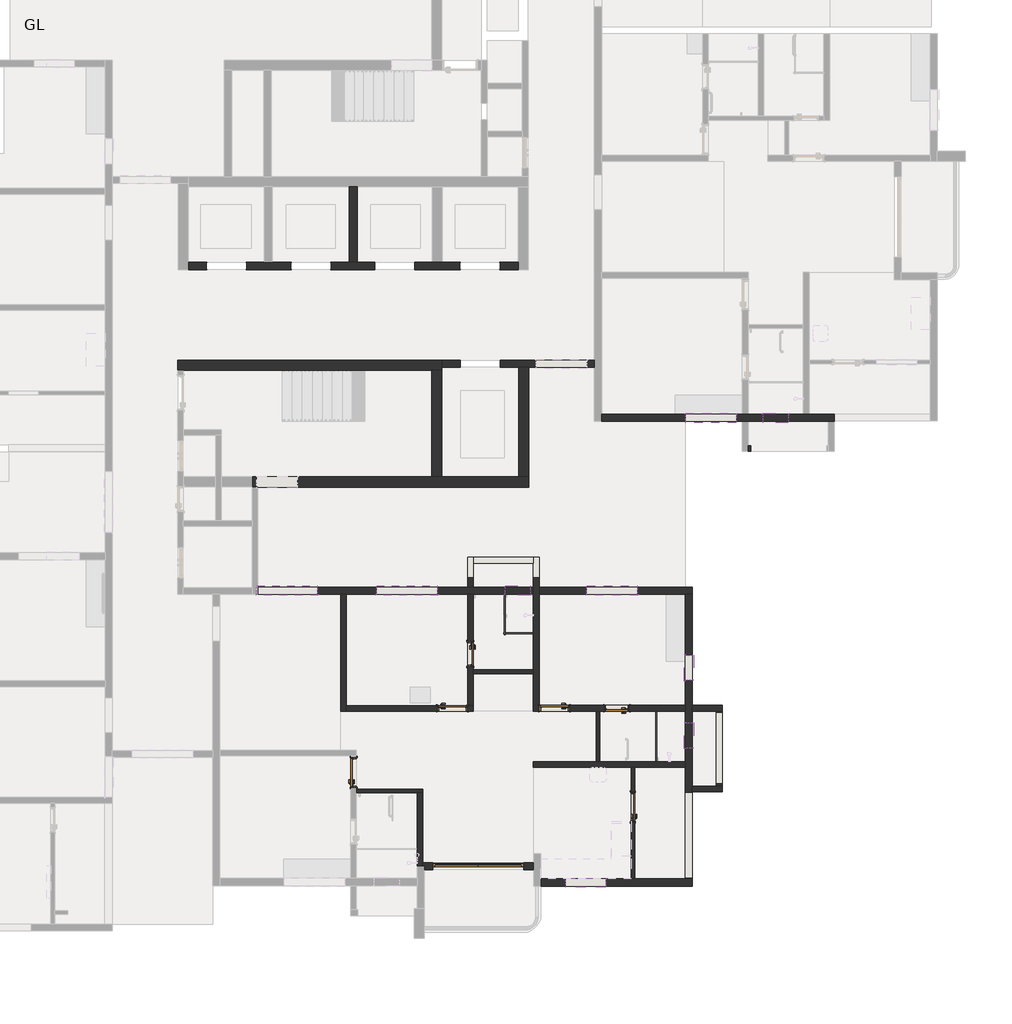
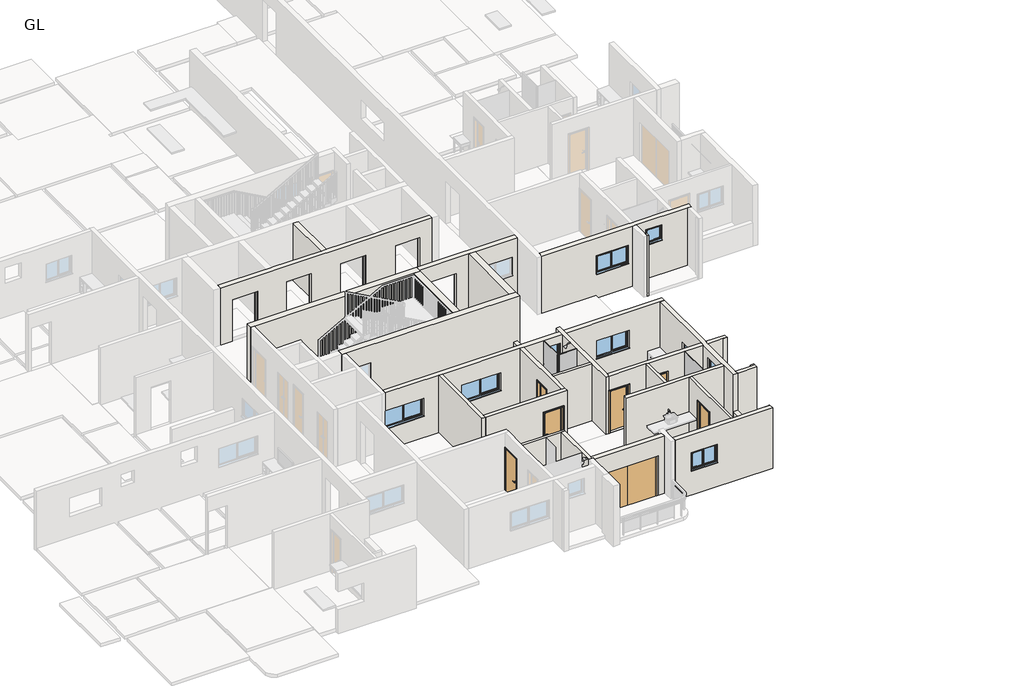
# One storey, part 4 of 14: 35 walls, 9 windows, 7 doors, 3 plates.
"""IFC4 building model written with IfcOpenShell, lengths in millimetres."""

from ifc_helpers import new_model, si_unit, frame, origin, origin_with_axes, place, context, project, spatial, polyline, outline, extrude, faceted_brep, transform, mapped, element, save
from components import doors_concept_extdbl_9_dbcc4ac8, doors_intsgl_2_5_door_ce04bd24, doors_intsgl_3_door_8261d8fb, doors_intsgl_3_door_f61d7fb9, doors_intsgl_3_door_feb48a3d, doors_intsgl_3_door_d2de26da, system_panel_glazed_00f127ae, system_panel_glazed_ff4fe8f0, system_panel_glazed_94d7f8cb, windows_dbl_plain_2_5_f94f9a84, windows_dbl_plain_4_905afcad, windows_dbl_plain_5_907a13a5, windows_dbl_plain_6_3da2432f, windows_sgl_plain_2_5_21186da1

model = new_model("IFC4")

# Units and contexts
model_context = context("Model", 3, world=origin())
ifc_project = project(units=[si_unit("LENGTHUNIT", "METRE", prefix="MILLI")], contexts=[model_context])

# Site, building, storey
site = spatial("IfcSite", under=ifc_project)
building = spatial("IfcBuilding", under=site)
storey = spatial("IfcBuildingStorey", under=building, Name="GL", Elevation=0.0)

# Doors
placement = place(None, origin())
doors_concept_extdbl_9_shape = doors_concept_extdbl_9_dbcc4ac8(model_context)
element("IfcDoor", 1, ObjectType="Doors_Concept_ExtDbl : 9'", at=placement, inside=storey, context=model_context, shape_type="MappedRepresentation", body=[
    mapped(doors_concept_extdbl_9_shape, transform((5777.5463567, 58086.1033045, 0.0), x_axis=(1.0, 0.0, 0.0), y_axis=(0.0, 1.0, 0.0), z_axis=(0.0, 0.0, 1.0))),
])
doors_intsgl_2_5_door_shape = doors_intsgl_2_5_door_ce04bd24(model_context)
element("IfcDoor", 2, ObjectType="Doors_IntSgl : 2.5' DOOR", at=placement, inside=storey, context=model_context, shape_type="MappedRepresentation", body=[
    mapped(doors_intsgl_2_5_door_shape, transform((5542.845694, 64510.7496197, 149.9616), x_axis=(0.0, -1.0, 0.0), y_axis=(1.0, 0.0, 0.0), z_axis=(0.0, 0.0, 1.0))),
])
element("IfcDoor", 3, ObjectType="Doors_IntSgl : 2.5' DOOR", at=placement, inside=storey, context=model_context, shape_type="MappedRepresentation", body=[
    mapped(doors_intsgl_2_5_door_shape, transform((9968.9401818, 62868.569994, 149.9616), x_axis=(-1.0, 0.0, 0.0), y_axis=(0.0, -1.0, 0.0), z_axis=(0.0, 0.0, 1.0))),
])
doors_intsgl_3_door_shape = doors_intsgl_3_door_8261d8fb(model_context)
element("IfcDoor", 4, ObjectType="Doors_IntSgl : 3' DOOR", at=placement, inside=storey, context=model_context, shape_type="MappedRepresentation", body=[
    mapped(doors_intsgl_3_door_shape, transform((8080.813694, 62868.569994, 149.9616), x_axis=(-1.0, 0.0, 0.0), y_axis=(0.0, -1.0, 0.0), z_axis=(0.0, 0.0, 1.0))),
])
doors_intsgl_3_door_2_shape = doors_intsgl_3_door_f61d7fb9(model_context)
element("IfcDoor", 5, ObjectType="Doors_IntSgl : 3' DOOR", at=placement, inside=storey, context=model_context, shape_type="MappedRepresentation", body=[
    mapped(doors_intsgl_3_door_2_shape, transform((4998.777694, 62865.3348421, 149.9616), x_axis=(1.0, 0.0, 0.0), y_axis=(0.0, 1.0, 0.0), z_axis=(0.0, 0.0, 1.0))),
])
doors_intsgl_3_door_3_shape = doors_intsgl_3_door_feb48a3d(model_context)
element("IfcDoor", 6, ObjectType="Doors_IntSgl : 3' DOOR", at=placement, inside=storey, context=model_context, shape_type="MappedRepresentation", body=[
    mapped(doors_intsgl_3_door_3_shape, transform((2014.4093567, 60927.6425384, 149.9616), x_axis=(0.0, 1.0, 0.0), y_axis=(-1.0, 0.0, 0.0), z_axis=(0.0, 0.0, 1.0))),
])
doors_intsgl_3_door_4_shape = doors_intsgl_3_door_d2de26da(model_context)
element("IfcDoor", 7, ObjectType="Doors_IntSgl : 3' DOOR", at=placement, inside=storey, context=model_context, shape_type="MappedRepresentation", body=[
    mapped(doors_intsgl_3_door_4_shape, transform((10458.253694, 59886.101994, 149.9616), x_axis=(0.0, 1.0, 0.0), y_axis=(-1.0, 0.0, 0.0), z_axis=(0.0, 0.0, 1.0))),
])

# Plates
system_panel_glazed_shape = system_panel_glazed_00f127ae(model_context)
element("IfcPlate", 8, ObjectType="System Panel : Glazed", at=placement, inside=storey, context=model_context, shape_type="MappedRepresentation", body=[
    mapped(system_panel_glazed_shape, transform((6544.913694, 65695.8028421, 0.0), x_axis=(0.0, -1.0, 0.0), y_axis=(1.0, 0.0, 0.0), z_axis=(0.0, 0.0, 1.0))),
])
system_panel_glazed_2_shape = system_panel_glazed_ff4fe8f0(model_context)
element("IfcPlate", 9, ObjectType="System Panel : Glazed", at=placement, inside=storey, context=model_context, shape_type="MappedRepresentation", body=[
    mapped(system_panel_glazed_2_shape, transform((6997.395694, 65098.9028421, 0.0), x_axis=(1.0, 0.0, 0.0), y_axis=(0.0, 1.0, 0.0), z_axis=(0.0, 0.0, 1.0))),
])
system_panel_glazed_3_shape = system_panel_glazed_94d7f8cb(model_context)
element("IfcPlate", 10, ObjectType="System Panel : Glazed", at=placement, inside=storey, context=model_context, shape_type="MappedRepresentation", body=[
    mapped(system_panel_glazed_3_shape, transform((11125.003694, 62017.669994, 0.0), x_axis=(0.0, -1.0, 0.0), y_axis=(1.0, 0.0, 0.0), z_axis=(0.0, 0.0, 1.0))),
])

# Walls
element("IfcWall", 11, ObjectType="W2", at=placement, inside=storey, context=model_context, shape_type="SweptSolid", body=[
    extrude(outline(polyline([(13943.8163556, 70812.6678957), (14020.0163556, 70812.6678957), (14020.0163556, 70638.9318957), (13943.8163556, 70638.9318957), (13943.8163556, 70812.6678957)])), origin_with_axes(), (0.0, 0.0, 1.0), 3000.0),
])
element("IfcWall", 12, ObjectType="W2", at=placement, inside=storey, context=model_context, shape_type="Brep", body=[
    faceted_brep([(3929.8233567, 60310.5083045, 0.0), (3929.8233567, 58086.1033045, 0.0), (3929.8233567, 58086.1033045, 3000.0), (3929.8233567, 60310.5083045, 3000.0), (4103.5593567, 60310.5083045, 0.0), (4103.5593567, 60310.5083045, 3000.0), (4103.5593567, 58192.7833045, 3000.0), (4103.5593567, 58086.1033045, 3000.0), (4103.5593567, 58086.1033045, 0.0), (4103.5593567, 58192.7833045, 0.0)], [[[0, 1, 2, 3]], [[4, 5, 6, 7, 8, 9]], [[1, 0, 4, 9, 8]], [[2, 1, 8, 7]], [[3, 2, 7, 6, 5]], [[0, 3, 5, 4]]]),
])
element("IfcWall", 13, ObjectType="W2", at=placement, inside=storey, context=model_context, shape_type="Brep", body=[
    faceted_brep([(1620.577694, 66317.7028421, 0.0), (1620.577694, 62778.4668421, 0.0), (1620.577694, 62778.4668421, 3000.0), (1620.577694, 66317.7028421, 3000.0), (1794.313694, 66317.7028421, 0.0), (1794.313694, 66317.7028421, 3000.0), (1794.313694, 62952.2028421, 3000.0), (1794.313694, 62778.4668421, 3000.0), (1794.313694, 62778.4668421, 0.0), (1794.313694, 62952.2028421, 0.0)], [[[0, 1, 2, 3]], [[4, 5, 6, 7, 8, 9]], [[1, 0, 4, 9, 8]], [[3, 2, 7, 6, 5]], [[0, 3, 5, 4]], [[2, 1, 8, 7]]]),
])
element("IfcWall", 14, ObjectType="W2", at=placement, inside=storey, context=model_context, shape_type="Brep", body=[
    faceted_brep([(1794.313694, 62778.4668421, 0.0), (5629.713694, 62778.4668421, 0.0), (5629.713694, 62778.4668421, 3000.0), (1794.313694, 62778.4668421, 3000.0), (5455.977694, 62778.4668421, 2259.9616), (5455.977694, 62778.4668421, 149.9616), (4541.577694, 62778.4668421, 149.9616), (4541.577694, 62778.4668421, 2259.9616), (5629.713694, 62952.2028421, 0.0), (5455.977694, 62952.2028421, 0.0), (1794.313694, 62952.2028421, 0.0), (1794.313694, 62952.2028421, 3000.0), (5455.977694, 62952.2028421, 3000.0), (5629.713694, 62952.2028421, 3000.0), (5455.977694, 62952.2028421, 149.9616), (5455.977694, 62952.2028421, 2259.9616), (4541.577694, 62952.2028421, 2259.9616), (4541.577694, 62952.2028421, 149.9616)], [[[0, 1, 2, 3], [4, 5, 6, 7]], [[8, 9, 10, 11, 12, 13], [14, 15, 16, 17]], [[1, 0, 10, 9, 8]], [[3, 2, 13, 12, 11]], [[0, 3, 11, 10]], [[2, 1, 8, 13]], [[14, 5, 4, 15]], [[15, 4, 7, 16]], [[16, 7, 6, 17]], [[5, 14, 17, 6]]]),
])
element("IfcWall", 15, ObjectType="W2", at=placement, inside=storey, context=model_context, shape_type="Brep", body=[
    faceted_brep([(5629.713694, 62952.2028421, 0.0), (5629.713694, 63913.8496197, 0.0), (5629.713694, 64028.1496197, 0.0), (5629.713694, 66317.7028421, 0.0), (5629.713694, 66317.7028421, 3000.0), (5629.713694, 64028.1496197, 3000.0), (5629.713694, 63913.8496197, 3000.0), (5629.713694, 62952.2028421, 3000.0), (5629.713694, 64129.7496197, 149.9616), (5629.713694, 64129.7496197, 2259.9616), (5629.713694, 64891.7496197, 2259.9616), (5629.713694, 64891.7496197, 149.9616), (5455.977694, 66317.7028421, 0.0), (5455.977694, 62952.2028421, 0.0), (5455.977694, 62952.2028421, 149.9616), (5455.977694, 62952.2028421, 2259.9616), (5455.977694, 62952.2028421, 3000.0), (5455.977694, 66317.7028421, 3000.0), (5455.977694, 64129.7496197, 2259.9616), (5455.977694, 64129.7496197, 149.9616), (5455.977694, 64891.7496197, 149.9616), (5455.977694, 64891.7496197, 2259.9616)], [[[0, 1, 2, 3, 4, 5, 6, 7], [8, 9, 10, 11]], [[12, 13, 14, 15, 16, 17], [18, 19, 20, 21]], [[3, 2, 1, 0, 13, 12]], [[7, 6, 5, 4, 17, 16]], [[0, 7, 16, 15, 14, 13]], [[4, 3, 12, 17]], [[8, 19, 18, 9]], [[9, 18, 21, 10]], [[10, 21, 20, 11]], [[19, 8, 11, 20]]]),
])
element("IfcWall", 16, ObjectType="W2", at=placement, inside=storey, context=model_context, shape_type="Brep", body=[
    faceted_brep([(5629.713694, 66531.0628421, 0.0), (5629.713694, 66823.1628421, 0.0), (5629.713694, 66823.1628421, 561.6), (5629.713694, 66823.1628421, 3000.0), (5629.713694, 66531.0628421, 3000.0), (5455.977694, 66531.0628421, 0.0), (5455.977694, 66531.0628421, 3000.0), (5455.977694, 66823.1628421, 3000.0), (5455.977694, 66823.1628421, 561.6), (5455.977694, 66823.1628421, 0.0)], [[[0, 1, 2, 3, 4]], [[5, 6, 7, 8, 9]], [[1, 0, 5, 9]], [[3, 2, 1, 9, 8, 7]], [[4, 3, 7, 6]], [[0, 4, 6, 5]]]),
])
element("IfcWall", 17, ObjectType="W2", at=placement, inside=storey, context=model_context, shape_type="Brep", body=[
    faceted_brep([(7623.613694, 62781.701994, 0.0), (7623.613694, 62955.437994, 0.0), (7623.613694, 66823.1628421, 0.0), (7623.613694, 66823.1628421, 561.6), (7623.613694, 66823.1628421, 3000.0), (7623.613694, 62955.437994, 3000.0), (7623.613694, 62781.701994, 3000.0), (7623.613694, 62781.701994, 2259.9616), (7623.613694, 62781.701994, 149.9616), (7449.877694, 62781.701994, 0.0), (7449.877694, 62781.701994, 3000.0), (7449.877694, 63913.8496197, 3000.0), (7449.877694, 64028.1496197, 3000.0), (7449.877694, 66823.1628421, 3000.0), (7449.877694, 66823.1628421, 561.6), (7449.877694, 66823.1628421, 0.0), (7449.877694, 64028.1496197, 0.0), (7449.877694, 63913.8496197, 0.0)], [[[0, 1, 2, 3, 4, 5, 6, 7, 8]], [[9, 10, 11, 12, 13, 14, 15, 16, 17]], [[2, 1, 0, 9, 17, 16, 15]], [[4, 3, 2, 15, 14, 13]], [[6, 5, 4, 13, 12, 11, 10]], [[0, 8, 7, 6, 10, 9]]]),
])
element("IfcWall", 18, ObjectType="W2", at=placement, inside=storey, context=model_context, shape_type="SweptSolid", body=[
    extrude(outline(polyline([(7449.877694, 67257.1218421), (5629.713694, 67257.1218421), (5629.713694, 67430.8578421), (7449.877694, 67430.8578421), (7449.877694, 67257.1218421)])), origin_with_axes(), (0.0, 0.0, 1.0), 561.6),
])
element("IfcWall", 19, ObjectType="W2", at=placement, inside=storey, context=model_context, shape_type="Brep", body=[
    faceted_brep([(5629.713694, 66823.1628421, 0.0), (5629.713694, 67257.1218421, 0.0), (5629.713694, 67430.8578421, 0.0), (5629.713694, 67430.8578421, 561.6), (5629.713694, 67257.1218421, 561.6), (5629.713694, 66823.1628421, 561.6), (5455.977694, 66823.1628421, 0.0), (5455.977694, 66823.1628421, 561.6), (5455.977694, 67430.8578421, 561.6), (5455.977694, 67430.8578421, 0.0)], [[[0, 1, 2, 3, 4, 5]], [[6, 7, 8, 9]], [[2, 1, 0, 6, 9]], [[5, 4, 3, 8, 7]], [[0, 5, 7, 6]], [[3, 2, 9, 8]]]),
])
element("IfcWall", 20, ObjectType="W2", at=placement, inside=storey, context=model_context, shape_type="Brep", body=[
    faceted_brep([(7623.613694, 66823.1628421, 0.0), (7623.613694, 67430.8578421, 0.0), (7623.613694, 67430.8578421, 561.6), (7623.613694, 66823.1628421, 561.6), (7449.877694, 66823.1628421, 0.0), (7449.877694, 66823.1628421, 561.6), (7449.877694, 67257.1218421, 561.6), (7449.877694, 67430.8578421, 561.6), (7449.877694, 67430.8578421, 0.0), (7449.877694, 67257.1218421, 0.0)], [[[0, 1, 2, 3]], [[4, 5, 6, 7, 8, 9]], [[1, 0, 4, 9, 8]], [[3, 2, 7, 6, 5]], [[0, 3, 5, 4]], [[2, 1, 8, 7]]]),
])
element("IfcWall", 21, ObjectType="W2", at=placement, inside=storey, context=model_context, shape_type="Brep", body=[
    faceted_brep([(12252.763694, 60342.3528421, 0.0), (13154.463694, 60342.3528421, 0.0), (13154.463694, 60342.3528421, 3000.0), (12252.763694, 60342.3528421, 3000.0), (12252.763694, 60516.0888421, 0.0), (12252.763694, 60516.0888421, 3000.0), (12980.727694, 60516.0888421, 3000.0), (13154.463694, 60516.0888421, 3000.0), (13154.463694, 60516.0888421, 0.0), (12980.727694, 60516.0888421, 0.0)], [[[0, 1, 2, 3]], [[4, 5, 6, 7, 8, 9]], [[1, 0, 4, 9, 8]], [[3, 2, 7, 6, 5]], [[2, 1, 8, 7]], [[0, 3, 5, 4]]]),
])
element("IfcWall", 22, ObjectType="W2", at=placement, inside=storey, context=model_context, shape_type="Brep", body=[
    faceted_brep([(12252.763694, 62781.701994, 0.0), (12980.727694, 62781.701994, 0.0), (13154.463694, 62781.701994, 0.0), (13154.463694, 62781.701994, 3000.0), (12980.727694, 62781.701994, 3000.0), (12252.763694, 62781.701994, 3000.0), (12252.763694, 62955.437994, 0.0), (12252.763694, 62955.437994, 3000.0), (13154.463694, 62955.437994, 3000.0), (13154.463694, 62955.437994, 0.0)], [[[0, 1, 2, 3, 4, 5]], [[6, 7, 8, 9]], [[2, 1, 0, 6, 9]], [[5, 4, 3, 8, 7]], [[0, 5, 7, 6]], [[3, 2, 9, 8]]]),
])
element("IfcWall", 23, ObjectType="W2", at=placement, inside=storey, context=model_context, shape_type="Brep", body=[
    faceted_brep([(13154.463694, 60516.0888421, 0.0), (13154.463694, 60592.2888421, 0.0), (13154.463694, 60592.2888421, 1171.2), (13154.463694, 60592.2888421, 3000.0), (13154.463694, 60516.0888421, 3000.0), (12980.727694, 60516.0888421, 0.0), (12980.727694, 60516.0888421, 3000.0), (12980.727694, 60592.2888421, 3000.0), (12980.727694, 60592.2888421, 1171.2), (12980.727694, 60592.2888421, 0.0)], [[[0, 1, 2, 3, 4]], [[5, 6, 7, 8, 9]], [[1, 0, 5, 9]], [[3, 2, 1, 9, 8, 7]], [[4, 3, 7, 6]], [[0, 4, 6, 5]]]),
])
element("IfcWall", 24, ObjectType="W2", at=placement, inside=storey, context=model_context, shape_type="SweptSolid", body=[
    extrude(outline(polyline([(13154.463694, 62756.301994), (13154.463694, 60592.2888421), (12980.727694, 60592.2888421), (12980.727694, 62756.301994), (13154.463694, 62756.301994)])), origin_with_axes(), (0.0, 0.0, 1.0), 1171.2),
])
element("IfcWall", 25, ObjectType="W2", at=placement, inside=storey, context=model_context, shape_type="Brep", body=[
    faceted_brep([(13154.463694, 62756.301994, 0.0), (13154.463694, 62781.701994, 0.0), (13154.463694, 62781.701994, 3000.0), (13154.463694, 62756.301994, 3000.0), (13154.463694, 62756.301994, 1171.2), (12980.727694, 62756.301994, 0.0), (12980.727694, 62756.301994, 1171.2), (12980.727694, 62756.301994, 3000.0), (12980.727694, 62781.701994, 3000.0), (12980.727694, 62781.701994, 0.0)], [[[0, 1, 2, 3, 4]], [[5, 6, 7, 8, 9]], [[1, 0, 5, 9]], [[3, 2, 8, 7]], [[0, 4, 3, 7, 6, 5]], [[2, 1, 9, 8]]]),
])
element("IfcWall", 26, ObjectType="W2", at=placement, inside=storey, context=model_context, shape_type="Brep", body=[
    faceted_brep([(12039.403694, 62955.437994, 0.0), (7623.613694, 62955.437994, 0.0), (7623.613694, 62955.437994, 149.9616), (8538.013694, 62955.437994, 149.9616), (8538.013694, 62955.437994, 2259.9616), (7623.613694, 62955.437994, 2259.9616), (7623.613694, 62955.437994, 3000.0), (12039.403694, 62955.437994, 3000.0), (9587.9401818, 62955.437994, 2259.9616), (9587.9401818, 62955.437994, 149.9616), (10349.9401818, 62955.437994, 149.9616), (10349.9401818, 62955.437994, 2259.9616), (7623.613694, 62781.701994, 0.0), (9346.6401818, 62781.701994, 0.0), (9460.9401818, 62781.701994, 0.0), (12039.403694, 62781.701994, 0.0), (12039.403694, 62781.701994, 3000.0), (9460.9401818, 62781.701994, 3000.0), (9346.6401818, 62781.701994, 3000.0), (7623.613694, 62781.701994, 3000.0), (7623.613694, 62781.701994, 2259.9616), (8538.013694, 62781.701994, 2259.9616), (8538.013694, 62781.701994, 149.9616), (7623.613694, 62781.701994, 149.9616), (9587.9401818, 62781.701994, 149.9616), (9587.9401818, 62781.701994, 2259.9616), (10349.9401818, 62781.701994, 2259.9616), (10349.9401818, 62781.701994, 149.9616)], [[[0, 1, 2, 3, 4, 5, 6, 7], [8, 9, 10, 11]], [[12, 13, 14, 15, 16, 17, 18, 19, 20, 21, 22, 23], [24, 25, 26, 27]], [[1, 0, 15, 14, 13, 12]], [[7, 6, 19, 18, 17, 16]], [[0, 7, 16, 15]], [[1, 12, 23, 2]], [[19, 6, 5, 20]], [[4, 21, 20, 5]], [[3, 22, 21, 4]], [[22, 3, 2, 23]], [[24, 9, 8, 25]], [[25, 8, 11, 26]], [[26, 11, 10, 27]], [[9, 24, 27, 10]]]),
])
element("IfcWall", 27, ObjectType="W2", at=placement, inside=storey, context=model_context, shape_type="Brep", body=[
    faceted_brep([(12039.403694, 61253.637994, 0.0), (9460.9401818, 61253.637994, 0.0), (9346.6401818, 61253.637994, 0.0), (7442.003694, 61253.637994, 0.0), (7442.003694, 61253.637994, 3000.0), (9346.6401818, 61253.637994, 3000.0), (9460.9401818, 61253.637994, 3000.0), (12039.403694, 61253.637994, 3000.0), (12039.403694, 61079.901994, 0.0), (12039.403694, 61079.901994, 3000.0), (10515.403694, 61079.901994, 3000.0), (10401.103694, 61079.901994, 3000.0), (7442.003694, 61079.901994, 3000.0), (7442.003694, 61079.901994, 0.0), (10401.103694, 61079.901994, 0.0), (10515.403694, 61079.901994, 0.0)], [[[0, 1, 2, 3, 4, 5, 6, 7]], [[8, 9, 10, 11, 12, 13, 14, 15]], [[3, 2, 1, 0, 8, 15, 14, 13]], [[4, 3, 13, 12]], [[7, 6, 5, 4, 12, 11, 10, 9]], [[0, 7, 9, 8]]]),
])
element("IfcWall", 28, ObjectType="W3", at=placement, inside=storey, context=model_context, shape_type="Brep", body=[
    faceted_brep([(2098.2293567, 60310.5083045, 0.0), (3929.8233567, 60310.5083045, 0.0), (4103.5593567, 60310.5083045, 0.0), (4103.5593567, 60310.5083045, 3000.0), (3929.8233567, 60310.5083045, 3000.0), (2098.2293567, 60310.5083045, 3000.0), (2098.2293567, 60424.8083045, 0.0), (2098.2293567, 60424.8083045, 3000.0), (4103.5593567, 60424.8083045, 3000.0), (4103.5593567, 60424.8083045, 0.0)], [[[0, 1, 2, 3, 4, 5]], [[6, 7, 8, 9]], [[2, 1, 0, 6, 9]], [[5, 4, 3, 8, 7]], [[0, 5, 7, 6]], [[3, 2, 9, 8]]]),
])
element("IfcWall", 29, ObjectType="W3", at=placement, inside=storey, context=model_context, shape_type="SweptSolid", body=[
    extrude(outline(polyline([(7449.877694, 63913.8496197), (5629.713694, 63913.8496197), (5629.713694, 64028.1496197), (7449.877694, 64028.1496197), (7449.877694, 63913.8496197)])), origin_with_axes(), (0.0, 0.0, 1.0), 3000.0),
])
element("IfcWall", 30, ObjectType="W3", at=placement, inside=storey, context=model_context, shape_type="SweptSolid", body=[
    extrude(outline(polyline([(9346.6401818, 61253.637994), (9346.6401818, 62781.701994), (9460.9401818, 62781.701994), (9460.9401818, 61253.637994), (9346.6401818, 61253.637994)])), origin_with_axes(), (0.0, 0.0, 1.0), 3000.0),
])
element("IfcWall", 31, ObjectType="W3", at=placement, inside=storey, context=model_context, shape_type="SweptSolid", body=[
    extrude(outline(polyline([(61079.901994, 0.0), (57707.6433045, 0.0), (57707.6433045, 3000.0), (61079.901994, 3000.0), (61079.901994, 0.0)]), holes=[polyline([(60343.301994, 149.9616), (60343.301994, 2259.9616), (59428.901994, 2259.9616), (59428.901994, 149.9616), (60343.301994, 149.9616)])]), frame((10401.103694, 0.0, 0.0), z_axis=(1.0, 0.0, 0.0), x_axis=(0.0, 1.0, 0.0)), (0.0, 0.0, 1.0), 114.3),
])
element("IfcWall", 32, ObjectType="W4", at=placement, inside=storey, context=model_context, shape_type="Brep", body=[
    faceted_brep([(-3305.0047841, 73095.6178911, 0.0), (-3137.3647841, 73095.6178911, 0.0), (4372.114024, 73095.6178911, 0.0), (4676.914024, 73095.6178911, 0.0), (4676.914024, 73095.6178911, 3000.0), (4372.114024, 73095.6178911, 3000.0), (-3137.3647841, 73095.6178911, 3000.0), (-3305.0047841, 73095.6178911, 3000.0), (-3305.0047841, 73400.4178911, 0.0), (-3305.0047841, 73400.4178911, 3000.0), (4676.914024, 73400.4178911, 3000.0), (4676.914024, 73400.4178911, 0.0), (4676.914024, 73177.9138911, 0.0), (4676.914024, 73177.9138911, 3000.0)], [[[0, 1, 2, 3, 4, 5, 6, 7]], [[8, 9, 10, 11]], [[3, 2, 1, 0, 8, 11, 12]], [[7, 6, 5, 4, 13, 10, 9]], [[4, 3, 12, 11, 10, 13]], [[0, 7, 9, 8]]]),
])
element("IfcWall", 33, ObjectType="W4", at=placement, inside=storey, context=model_context, shape_type="SweptSolid", body=[
    extrude(outline(polyline([(4372.114024, 69866.1033979), (4372.114024, 73095.6178911), (4676.914024, 73095.6178911), (4676.914024, 69866.1033979), (4372.114024, 69866.1033979)])), origin_with_axes(), (0.0, 0.0, 1.0), 3000.0),
])
element("IfcWall", 34, ObjectType="W4", at=placement, inside=storey, context=model_context, shape_type="Brep", body=[
    faceted_brep([(7306.113694, 69866.1033979, 0.0), (7001.313694, 69866.1033979, 0.0), (4676.914024, 69866.1033979, 0.0), (4372.114024, 69866.1033979, 0.0), (-1053.026306, 69866.1033979, 0.0), (-1053.026306, 69866.1033979, 3000.0), (4372.114024, 69866.1033979, 3000.0), (4676.914024, 69866.1033979, 3000.0), (7001.313694, 69866.1033979, 3000.0), (7306.113694, 69866.1033979, 3000.0), (308.413694, 69866.1033979, 2110.0), (-910.786306, 69866.1033979, 2110.0), (-910.786306, 69866.1033979, 1200.0), (308.413694, 69866.1033979, 1200.0), (7306.113694, 69561.3033979, 0.0), (7306.113694, 69561.3033979, 3000.0), (-885.386306, 69561.3033979, 3000.0), (-1053.026306, 69561.3033979, 3000.0), (-1053.026306, 69561.3033979, 0.0), (-885.386306, 69561.3033979, 0.0), (308.413694, 69561.3033979, 2110.0), (308.413694, 69561.3033979, 1200.0), (-910.786306, 69561.3033979, 1200.0), (-910.786306, 69561.3033979, 2110.0), (-1053.026306, 69566.3628421, 0.0), (-1053.026306, 69566.3628421, 3000.0)], [[[0, 1, 2, 3, 4, 5, 6, 7, 8, 9], [10, 11, 12, 13]], [[14, 15, 16, 17, 18, 19], [20, 21, 22, 23]], [[4, 3, 2, 1, 0, 14, 19, 18, 24]], [[9, 8, 7, 6, 5, 25, 17, 16, 15]], [[0, 9, 15, 14]], [[5, 4, 24, 18, 17, 25]], [[21, 20, 10, 13]], [[22, 21, 13, 12]], [[23, 22, 12, 11]], [[20, 23, 11, 10]]]),
])
element("IfcWall", 35, ObjectType="W4", at=placement, inside=storey, context=model_context, shape_type="SweptSolid", body=[
    extrude(outline(polyline([(7306.113694, 73177.9138911), (7306.113694, 69866.1033979), (7001.313694, 69866.1033979), (7001.313694, 73177.9138911), (7306.113694, 73177.9138911)])), origin_with_axes(), (0.0, 0.0, 1.0), 3000.0),
])
element("IfcWall", 36, ObjectType="W6", at=placement, inside=storey, context=model_context, shape_type="SweptSolid", body=[
    extrude(outline(polyline([(1881.4721554, 76353.9927724), (1881.4721554, 78643.5487724), (2125.3121554, 78643.5487724), (2125.3121554, 76353.9927724), (1881.4721554, 76353.9927724)])), origin_with_axes(), (0.0, 0.0, 1.0), 3000.0),
])
element("IfcWall", 37, ObjectType="W7", at=placement, inside=storey, context=model_context, shape_type="Brep", body=[
    faceted_brep([(6986.2068654, 76131.4887724, 3000.0), (-2983.2931346, 76131.4887724, 3000.0), (-2983.2931346, 76131.4887724, 0.0), (-2434.4804896, 76131.4887724, 0.0), (-2434.4804896, 76131.4887724, 2238.0), (-1235.2804896, 76131.4887724, 2238.0), (-1235.2804896, 76131.4887724, 0.0), (119.8221554, 76131.4887724, 0.0), (119.8221554, 76131.4887724, 2238.0), (1319.0221554, 76131.4887724, 2238.0), (1319.0221554, 76131.4887724, 0.0), (2654.4095104, 76131.4887724, 0.0), (2654.4095104, 76131.4887724, 2238.0), (3853.6095104, 76131.4887724, 2238.0), (3853.6095104, 76131.4887724, 0.0), (5237.2568654, 76131.4887724, 0.0), (5237.2568654, 76131.4887724, 2238.0), (6436.4568654, 76131.4887724, 2238.0), (6436.4568654, 76131.4887724, 0.0), (6986.2068654, 76131.4887724, 0.0), (-2983.2931346, 76353.9927724, 3000.0), (-686.4678446, 76353.9927724, 3000.0), (-442.6278446, 76353.9927724, 3000.0), (1881.4721554, 76353.9927724, 3000.0), (2125.3121554, 76353.9927724, 3000.0), (4382.7068654, 76353.9927724, 3000.0), (4687.5068654, 76353.9927724, 3000.0), (6986.2068654, 76353.9927724, 3000.0), (6986.2068654, 76353.9927724, 0.0), (6436.4568654, 76353.9927724, 0.0), (6436.4568654, 76353.9927724, 2238.0), (5237.2568654, 76353.9927724, 2238.0), (5237.2568654, 76353.9927724, 0.0), (4687.5068654, 76353.9927724, 0.0), (4382.7068654, 76353.9927724, 0.0), (3853.6095104, 76353.9927724, 0.0), (3853.6095104, 76353.9927724, 2238.0), (2654.4095104, 76353.9927724, 2238.0), (2654.4095104, 76353.9927724, 0.0), (2125.3121554, 76353.9927724, 0.0), (1881.4721554, 76353.9927724, 0.0), (1319.0221554, 76353.9927724, 0.0), (1319.0221554, 76353.9927724, 2238.0), (119.8221554, 76353.9927724, 2238.0), (119.8221554, 76353.9927724, 0.0), (-442.6278446, 76353.9927724, 0.0), (-686.4678446, 76353.9927724, 0.0), (-1235.2804896, 76353.9927724, 0.0), (-1235.2804896, 76353.9927724, 2238.0), (-2434.4804896, 76353.9927724, 2238.0), (-2434.4804896, 76353.9927724, 0.0), (-2983.2931346, 76353.9927724, 0.0), (-2434.4804896, 76337.4887724, 0.0), (-2444.4804896, 76337.4887724, 0.0), (-2444.4804896, 76151.4887724, 0.0), (-2434.4804896, 76151.4887724, 0.0), (6436.4568654, 76151.4887724, 0.0), (6446.4568654, 76151.4887724, 0.0), (6446.4568654, 76337.4887724, 0.0), (6436.4568654, 76337.4887724, 0.0), (-1235.2804896, 76151.4887724, 0.0), (-1225.2804896, 76151.4887724, 0.0), (-1225.2804896, 76337.4887724, 0.0), (-1235.2804896, 76337.4887724, 0.0), (119.8221554, 76337.4887724, 0.0), (109.8221554, 76337.4887724, 0.0), (109.8221554, 76151.4887724, 0.0), (119.8221554, 76151.4887724, 0.0), (1319.0221554, 76151.4887724, 0.0), (1329.0221554, 76151.4887724, 0.0), (1329.0221554, 76337.4887724, 0.0), (1319.0221554, 76337.4887724, 0.0), (2654.4095104, 76337.4887724, 0.0), (2644.4095104, 76337.4887724, 0.0), (2644.4095104, 76151.4887724, 0.0), (2654.4095104, 76151.4887724, 0.0), (3853.6095104, 76151.4887724, 0.0), (3863.6095104, 76151.4887724, 0.0), (3863.6095104, 76337.4887724, 0.0), (3853.6095104, 76337.4887724, 0.0), (5237.2568654, 76337.4887724, 0.0), (5227.2568654, 76337.4887724, 0.0), (5227.2568654, 76151.4887724, 0.0), (5237.2568654, 76151.4887724, 0.0), (-2434.4804896, 76151.4887724, 2238.0), (-1235.2804896, 76151.4887724, 2238.0), (-2434.4804896, 76337.4887724, 2238.0), (-1235.2804896, 76337.4887724, 2238.0), (-1225.2804896, 76337.4887724, 2248.0), (-2444.4804896, 76337.4887724, 2248.0), (-2444.4804896, 76151.4887724, 2248.0), (-1225.2804896, 76151.4887724, 2248.0), (119.8221554, 76151.4887724, 2238.0), (1319.0221554, 76151.4887724, 2238.0), (119.8221554, 76337.4887724, 2238.0), (1319.0221554, 76337.4887724, 2238.0), (1329.0221554, 76337.4887724, 2248.0), (109.8221554, 76337.4887724, 2248.0), (109.8221554, 76151.4887724, 2248.0), (1329.0221554, 76151.4887724, 2248.0), (2654.4095104, 76151.4887724, 2238.0), (3853.6095104, 76151.4887724, 2238.0), (2654.4095104, 76337.4887724, 2238.0), (3853.6095104, 76337.4887724, 2238.0), (3863.6095104, 76337.4887724, 2248.0), (2644.4095104, 76337.4887724, 2248.0), (2644.4095104, 76151.4887724, 2248.0), (3863.6095104, 76151.4887724, 2248.0), (5237.2568654, 76151.4887724, 2238.0), (6436.4568654, 76151.4887724, 2238.0), (5237.2568654, 76337.4887724, 2238.0), (6436.4568654, 76337.4887724, 2238.0), (6446.4568654, 76337.4887724, 2248.0), (5227.2568654, 76337.4887724, 2248.0), (5227.2568654, 76151.4887724, 2248.0), (6446.4568654, 76151.4887724, 2248.0)], [[[0, 1, 2, 3, 4, 5, 6, 7, 8, 9, 10, 11, 12, 13, 14, 15, 16, 17, 18, 19]], [[20, 21, 22, 23, 24, 25, 26, 27, 28, 29, 30, 31, 32, 33, 34, 35, 36, 37, 38, 39, 40, 41, 42, 43, 44, 45, 46, 47, 48, 49, 50, 51]], [[2, 51, 50, 52, 53, 54, 55, 3]], [[28, 19, 18, 56, 57, 58, 59, 29]], [[6, 60, 61, 62, 63, 47, 46, 45, 44, 64, 65, 66, 67, 7]], [[10, 68, 69, 70, 71, 41, 40, 39, 38, 72, 73, 74, 75, 11]], [[14, 76, 77, 78, 79, 35, 34, 33, 32, 80, 81, 82, 83, 15]], [[1, 0, 27, 26, 25, 24, 23, 22, 21, 20]], [[2, 1, 20, 51]], [[0, 19, 28, 27]], [[84, 4, 3, 55]], [[5, 85, 60, 6]], [[4, 84, 85, 5]], [[86, 87, 63, 62, 88, 89, 53, 52]], [[85, 84, 55, 54, 90, 91, 61, 60]], [[89, 90, 54, 53]], [[91, 88, 62, 61]], [[89, 88, 91, 90]], [[49, 86, 52, 50]], [[87, 48, 47, 63]], [[87, 86, 49, 48]], [[92, 8, 7, 67]], [[9, 93, 68, 10]], [[8, 92, 93, 9]], [[94, 95, 71, 70, 96, 97, 65, 64]], [[93, 92, 67, 66, 98, 99, 69, 68]], [[97, 98, 66, 65]], [[99, 96, 70, 69]], [[97, 96, 99, 98]], [[43, 94, 64, 44]], [[95, 42, 41, 71]], [[95, 94, 43, 42]], [[100, 12, 11, 75]], [[13, 101, 76, 14]], [[12, 100, 101, 13]], [[102, 103, 79, 78, 104, 105, 73, 72]], [[101, 100, 75, 74, 106, 107, 77, 76]], [[105, 106, 74, 73]], [[107, 104, 78, 77]], [[105, 104, 107, 106]], [[37, 102, 72, 38]], [[103, 36, 35, 79]], [[103, 102, 37, 36]], [[108, 16, 15, 83]], [[17, 109, 56, 18]], [[16, 108, 109, 17]], [[110, 111, 59, 58, 112, 113, 81, 80]], [[109, 108, 83, 82, 114, 115, 57, 56]], [[113, 114, 82, 81]], [[115, 112, 58, 57]], [[113, 112, 115, 114]], [[31, 110, 80, 32]], [[111, 30, 29, 59]], [[111, 110, 31, 30]]]),
])
element("IfcWall", 38, ObjectType="W7", at=placement, inside=storey, context=model_context, shape_type="Brep", body=[
    faceted_brep([(9294.7969726, 73177.9138911, 3000.0), (7306.113694, 73177.9138911, 3000.0), (7001.313694, 73177.9138911, 3000.0), (4676.914024, 73177.9138911, 3000.0), (4676.914024, 73177.9138911, 0.0), (5239.513859, 73177.9138911, 0.0), (5239.513859, 73177.9138911, 2238.0), (6438.713859, 73177.9138911, 2238.0), (6438.713859, 73177.9138911, 0.0), (7001.313694, 73177.9138911, 0.0), (7306.113694, 73177.9138911, 0.0), (9294.7969726, 73177.9138911, 0.0), (9062.4553333, 73177.9138911, 2110.0), (9062.4553333, 73177.9138911, 1200.0), (7538.4553333, 73177.9138911, 1200.0), (7538.4553333, 73177.9138911, 2110.0), (4676.914024, 73400.4178911, 3000.0), (9294.7969726, 73400.4178911, 3000.0), (9294.7969726, 73400.4178911, 0.0), (6438.713859, 73400.4178911, 0.0), (6438.713859, 73400.4178911, 2238.0), (5239.513859, 73400.4178911, 2238.0), (5239.513859, 73400.4178911, 0.0), (4676.914024, 73400.4178911, 0.0), (9062.4553333, 73400.4178911, 1200.0), (9062.4553333, 73400.4178911, 2110.0), (7538.4553333, 73400.4178911, 2110.0), (7538.4553333, 73400.4178911, 1200.0), (5239.513859, 73383.9138911, 0.0), (5229.513859, 73383.9138911, 0.0), (5229.513859, 73197.9138911, 0.0), (5239.513859, 73197.9138911, 0.0), (6438.713859, 73197.9138911, 0.0), (6448.713859, 73197.9138911, 0.0), (6448.713859, 73383.9138911, 0.0), (6438.713859, 73383.9138911, 0.0), (5239.513859, 73197.9138911, 2238.0), (6438.713859, 73197.9138911, 2238.0), (5239.513859, 73383.9138911, 2238.0), (6438.713859, 73383.9138911, 2238.0), (6448.713859, 73383.9138911, 2248.0), (5229.513859, 73383.9138911, 2248.0), (5229.513859, 73197.9138911, 2248.0), (6448.713859, 73197.9138911, 2248.0)], [[[0, 1, 2, 3, 4, 5, 6, 7, 8, 9, 10, 11], [12, 13, 14, 15]], [[16, 17, 18, 19, 20, 21, 22, 23], [24, 25, 26, 27]], [[4, 23, 22, 28, 29, 30, 31, 5]], [[18, 11, 10, 9, 8, 32, 33, 34, 35, 19]], [[3, 2, 1, 0, 17, 16]], [[4, 3, 16, 23]], [[0, 11, 18, 17]], [[13, 12, 25, 24]], [[14, 13, 24, 27]], [[15, 14, 27, 26]], [[12, 15, 26, 25]], [[36, 6, 5, 31]], [[7, 37, 32, 8]], [[6, 36, 37, 7]], [[38, 39, 35, 34, 40, 41, 29, 28]], [[37, 36, 31, 30, 42, 43, 33, 32]], [[41, 42, 30, 29]], [[43, 40, 34, 33]], [[41, 40, 43, 42]], [[21, 38, 28, 22]], [[39, 20, 19, 35]], [[39, 38, 21, 20]]]),
])
element("IfcWall", 39, ObjectType="W8", at=placement, inside=storey, context=model_context, shape_type="Brep", body=[
    faceted_brep([(9508.1569726, 71549.2678957, 0.0), (13770.0803556, 71549.2678957, 0.0), (13943.8163556, 71549.2678957, 0.0), (16370.2209726, 71549.2678957, 0.0), (16543.9569726, 71549.2678957, 0.0), (16543.9569726, 71549.2678957, 3000.0), (16370.2209726, 71549.2678957, 3000.0), (13943.8163556, 71549.2678957, 3000.0), (13770.0803556, 71549.2678957, 3000.0), (9508.1569726, 71549.2678957, 3000.0), (13583.0862029, 71549.2678957, 2110.0), (13583.0862029, 71549.2678957, 1200.0), (12059.0862029, 71549.2678957, 1200.0), (12059.0862029, 71549.2678957, 2110.0), (15157.8862029, 71549.2678957, 2590.8), (15157.8862029, 71549.2678957, 1828.8), (14395.8862029, 71549.2678957, 1828.8), (14395.8862029, 71549.2678957, 2590.8), (9508.1569726, 71762.6278957, 0.0), (9508.1569726, 71762.6278957, 3000.0), (13770.0803556, 71762.6278957, 3000.0), (13943.8163556, 71762.6278957, 3000.0), (15615.0862029, 71762.6278957, 3000.0), (15788.8222029, 71762.6278957, 3000.0), (16543.9569726, 71762.6278957, 3000.0), (16543.9569726, 71762.6278957, 0.0), (15788.8222029, 71762.6278957, 0.0), (15615.0862029, 71762.6278957, 0.0), (13943.8163556, 71762.6278957, 0.0), (13770.0803556, 71762.6278957, 0.0), (13583.0862029, 71762.6278957, 2110.0), (12059.0862029, 71762.6278957, 2110.0), (12059.0862029, 71762.6278957, 1200.0), (13583.0862029, 71762.6278957, 1200.0), (15157.8862029, 71762.6278957, 2590.8), (14395.8862029, 71762.6278957, 2590.8), (14395.8862029, 71762.6278957, 1828.8), (15157.8862029, 71762.6278957, 1828.8)], [[[0, 1, 2, 3, 4, 5, 6, 7, 8, 9], [10, 11, 12, 13], [14, 15, 16, 17]], [[18, 19, 20, 21, 22, 23, 24, 25, 26, 27, 28, 29], [30, 31, 32, 33], [34, 35, 36, 37]], [[4, 3, 2, 1, 0, 18, 29, 28, 27, 26, 25]], [[9, 8, 7, 6, 5, 24, 23, 22, 21, 20, 19]], [[0, 9, 19, 18]], [[5, 4, 25, 24]], [[11, 10, 30, 33]], [[12, 11, 33, 32]], [[13, 12, 32, 31]], [[10, 13, 31, 30]], [[15, 14, 34, 37]], [[16, 15, 37, 36]], [[17, 16, 36, 35]], [[14, 17, 35, 34]]]),
])
element("IfcWall", 40, ObjectType="W8", at=placement, inside=storey, context=model_context, shape_type="Brep", body=[
    faceted_brep([(-885.386306, 66317.7028421, 0.0), (1620.577694, 66317.7028421, 0.0), (1794.313694, 66317.7028421, 0.0), (5455.977694, 66317.7028421, 0.0), (5629.713694, 66317.7028421, 0.0), (12039.403694, 66317.7028421, 0.0), (12252.763694, 66317.7028421, 0.0), (12252.763694, 66317.7028421, 3000.0), (12039.403694, 66317.7028421, 3000.0), (5629.713694, 66317.7028421, 3000.0), (5455.977694, 66317.7028421, 3000.0), (1794.313694, 66317.7028421, 3000.0), (1620.577694, 66317.7028421, 3000.0), (-885.386306, 66317.7028421, 3000.0), (-885.386306, 66317.7028421, 2110.0), (918.013694, 66317.7028421, 2110.0), (918.013694, 66317.7028421, 1200.0), (-885.386306, 66317.7028421, 1200.0), (9067.603694, 66317.7028421, 2110.0), (10591.603694, 66317.7028421, 2110.0), (10591.603694, 66317.7028421, 1200.0), (9067.603694, 66317.7028421, 1200.0), (6594.913694, 66317.7028421, 2590.8), (7356.913694, 66317.7028421, 2590.8), (7356.913694, 66317.7028421, 1828.8), (6594.913694, 66317.7028421, 1828.8), (2710.745694, 66317.7028421, 2110.0), (4539.545694, 66317.7028421, 2110.0), (4539.545694, 66317.7028421, 1200.0), (2710.745694, 66317.7028421, 1200.0), (12252.763694, 66531.0628421, 0.0), (5629.713694, 66531.0628421, 0.0), (5455.977694, 66531.0628421, 0.0), (-885.386306, 66531.0628421, 0.0), (-885.386306, 66531.0628421, 1200.0), (918.013694, 66531.0628421, 1200.0), (918.013694, 66531.0628421, 2110.0), (-885.386306, 66531.0628421, 2110.0), (-885.386306, 66531.0628421, 3000.0), (5455.977694, 66531.0628421, 3000.0), (5629.713694, 66531.0628421, 3000.0), (12252.763694, 66531.0628421, 3000.0), (9067.603694, 66531.0628421, 2110.0), (9067.603694, 66531.0628421, 1200.0), (10591.603694, 66531.0628421, 1200.0), (10591.603694, 66531.0628421, 2110.0), (6594.913694, 66531.0628421, 2590.8), (6594.913694, 66531.0628421, 1828.8), (7356.913694, 66531.0628421, 1828.8), (7356.913694, 66531.0628421, 2590.8), (2710.745694, 66531.0628421, 2110.0), (2710.745694, 66531.0628421, 1200.0), (4539.545694, 66531.0628421, 1200.0), (4539.545694, 66531.0628421, 2110.0)], [[[0, 1, 2, 3, 4, 5, 6, 7, 8, 9, 10, 11, 12, 13, 14, 15, 16, 17], [18, 19, 20, 21], [22, 23, 24, 25], [26, 27, 28, 29]], [[30, 31, 32, 33, 34, 35, 36, 37, 38, 39, 40, 41], [42, 43, 44, 45], [46, 47, 48, 49], [50, 51, 52, 53]], [[6, 5, 4, 3, 2, 1, 0, 33, 32, 31, 30]], [[13, 12, 11, 10, 9, 8, 7, 41, 40, 39, 38]], [[13, 38, 37, 14]], [[33, 0, 17, 34]], [[7, 6, 30, 41]], [[43, 42, 18, 21]], [[44, 43, 21, 20]], [[45, 44, 20, 19]], [[42, 45, 19, 18]], [[47, 46, 22, 25]], [[48, 47, 25, 24]], [[49, 48, 24, 23]], [[46, 49, 23, 22]], [[51, 50, 26, 29]], [[52, 51, 29, 28]], [[53, 52, 28, 27]], [[50, 53, 27, 26]], [[16, 35, 34, 17]], [[35, 16, 15, 36]], [[36, 15, 14, 37]]]),
])
element("IfcWall", 41, ObjectType="W8", at=placement, inside=storey, context=model_context, shape_type="Brep", body=[
    faceted_brep([(7149.1463567, 57979.4233045, 2110.0), (7149.1463567, 57979.4233045, 0.0), (7451.5333567, 57979.4233045, 0.0), (7451.5333567, 57979.4233045, 3000.0), (4143.1833567, 57979.4233045, 3000.0), (4143.1833567, 57979.4233045, 0.0), (4405.9463567, 57979.4233045, 0.0), (4405.9463567, 57979.4233045, 2110.0), (7451.5333567, 58192.7833045, 0.0), (7149.1463567, 58192.7833045, 0.0), (7149.1463567, 58192.7833045, 2110.0), (4405.9463567, 58192.7833045, 2110.0), (4405.9463567, 58192.7833045, 0.0), (4103.5593567, 58192.7833045, 0.0), (4103.5593567, 58192.7833045, 3000.0), (7451.5333567, 58192.7833045, 3000.0), (4143.1833567, 58086.1033045, 0.0), (4103.5593567, 58086.1033045, 0.0), (4103.5593567, 58086.1033045, 3000.0), (4143.1833567, 58086.1033045, 3000.0)], [[[0, 1, 2, 3, 4, 5, 6, 7]], [[8, 9, 10, 11, 12, 13, 14, 15]], [[6, 5, 16, 17, 13, 12]], [[2, 1, 9, 8]], [[4, 3, 15, 14, 18, 19]], [[5, 4, 19, 16]], [[19, 18, 17, 16]], [[18, 14, 13, 17]], [[3, 2, 8, 15]], [[12, 11, 7, 6]], [[10, 9, 1, 0]], [[11, 10, 0, 7]]]),
])
element("IfcWall", 42, ObjectType="W8", at=placement, inside=storey, context=model_context, shape_type="Brep", body=[
    faceted_brep([(7664.8933567, 57494.2833045, 0.0), (12252.763694, 57494.2833045, 0.0), (12252.763694, 57494.2833045, 3000.0), (7664.8933567, 57494.2833045, 3000.0), (9642.5985254, 57494.2833045, 2110.0), (9642.5985254, 57494.2833045, 1200.0), (8423.3985254, 57494.2833045, 1200.0), (8423.3985254, 57494.2833045, 2110.0), (7664.8933567, 57707.6433045, 0.0), (7664.8933567, 57707.6433045, 3000.0), (10401.103694, 57707.6433045, 3000.0), (10515.403694, 57707.6433045, 3000.0), (12039.403694, 57707.6433045, 3000.0), (12252.763694, 57707.6433045, 3000.0), (12252.763694, 57707.6433045, 0.0), (12039.403694, 57707.6433045, 0.0), (10515.403694, 57707.6433045, 0.0), (10401.103694, 57707.6433045, 0.0), (9642.5985254, 57707.6433045, 2110.0), (8423.3985254, 57707.6433045, 2110.0), (8423.3985254, 57707.6433045, 1200.0), (9642.5985254, 57707.6433045, 1200.0)], [[[0, 1, 2, 3], [4, 5, 6, 7]], [[8, 9, 10, 11, 12, 13, 14, 15, 16, 17], [18, 19, 20, 21]], [[1, 0, 8, 17, 16, 15, 14]], [[3, 2, 13, 12, 11, 10, 9]], [[0, 3, 9, 8]], [[2, 1, 14, 13]], [[5, 4, 18, 21]], [[6, 5, 21, 20]], [[7, 6, 20, 19]], [[4, 7, 19, 18]]]),
])
element("IfcWall", 43, ObjectType="W8", at=placement, inside=storey, context=model_context, shape_type="Brep", body=[
    faceted_brep([(12039.403694, 66317.7028421, 0.0), (12039.403694, 62955.437994, 0.0), (12039.403694, 62781.701994, 0.0), (12039.403694, 61253.637994, 0.0), (12039.403694, 61079.901994, 0.0), (12039.403694, 60323.8433045, 0.0), (12039.403694, 60323.8433045, 1171.2), (12039.403694, 60323.8433045, 3000.0), (12039.403694, 61079.901994, 3000.0), (12039.403694, 61253.637994, 3000.0), (12039.403694, 62781.701994, 3000.0), (12039.403694, 62955.437994, 3000.0), (12039.403694, 66317.7028421, 3000.0), (12039.403694, 62426.101994, 2590.8), (12039.403694, 61664.101994, 2590.8), (12039.403694, 61664.101994, 1828.8), (12039.403694, 62426.101994, 1828.8), (12039.403694, 64479.437994, 2110.0), (12039.403694, 63717.437994, 2110.0), (12039.403694, 63717.437994, 1200.0), (12039.403694, 64479.437994, 1200.0), (12252.763694, 66317.7028421, 0.0), (12252.763694, 66317.7028421, 3000.0), (12252.763694, 62955.437994, 3000.0), (12252.763694, 62781.701994, 3000.0), (12252.763694, 60516.0888421, 3000.0), (12252.763694, 60342.3528421, 3000.0), (12252.763694, 60323.8433045, 3000.0), (12252.763694, 60323.8433045, 1171.2), (12252.763694, 60323.8433045, 0.0), (12252.763694, 60342.3528421, 0.0), (12252.763694, 60516.0888421, 0.0), (12252.763694, 62781.701994, 0.0), (12252.763694, 62955.437994, 0.0), (12252.763694, 62426.101994, 2590.8), (12252.763694, 62426.101994, 1828.8), (12252.763694, 61664.101994, 1828.8), (12252.763694, 61664.101994, 2590.8), (12252.763694, 64479.437994, 2110.0), (12252.763694, 64479.437994, 1200.0), (12252.763694, 63717.437994, 1200.0), (12252.763694, 63717.437994, 2110.0)], [[[0, 1, 2, 3, 4, 5, 6, 7, 8, 9, 10, 11, 12], [13, 14, 15, 16], [17, 18, 19, 20]], [[21, 22, 23, 24, 25, 26, 27, 28, 29, 30, 31, 32, 33], [34, 35, 36, 37], [38, 39, 40, 41]], [[5, 4, 3, 2, 1, 0, 21, 33, 32, 31, 30, 29]], [[7, 6, 5, 29, 28, 27]], [[12, 11, 10, 9, 8, 7, 27, 26, 25, 24, 23, 22]], [[0, 12, 22, 21]], [[35, 34, 13, 16]], [[36, 35, 16, 15]], [[37, 36, 15, 14]], [[34, 37, 14, 13]], [[39, 38, 17, 20]], [[40, 39, 20, 19]], [[41, 40, 19, 18]], [[38, 41, 18, 17]]]),
])
element("IfcWall", 44, ObjectType="W8", at=placement, inside=storey, context=model_context, shape_type="SweptSolid", body=[
    extrude(outline(polyline([(12039.403694, 57733.0433045), (12039.403694, 60323.8433045), (12252.763694, 60323.8433045), (12252.763694, 57733.0433045), (12039.403694, 57733.0433045)])), origin_with_axes(), (0.0, 0.0, 1.0), 1171.2),
])
element("IfcWall", 45, ObjectType="W8", at=placement, inside=storey, context=model_context, shape_type="Brep", body=[
    faceted_brep([(12039.403694, 57733.0433045, 0.0), (12039.403694, 57707.6433045, 0.0), (12039.403694, 57707.6433045, 3000.0), (12039.403694, 57733.0433045, 3000.0), (12039.403694, 57733.0433045, 1171.2), (12252.763694, 57733.0433045, 0.0), (12252.763694, 57733.0433045, 1171.2), (12252.763694, 57733.0433045, 3000.0), (12252.763694, 57707.6433045, 3000.0), (12252.763694, 57707.6433045, 0.0)], [[[0, 1, 2, 3, 4]], [[5, 6, 7, 8, 9]], [[1, 0, 5, 9]], [[3, 2, 8, 7]], [[0, 4, 3, 7, 6, 5]], [[2, 1, 9, 8]]]),
])

# Windows
windows_dbl_plain_2_5_shape = windows_dbl_plain_2_5_f94f9a84(model_context)
element("IfcWindow", 46, ObjectType="Windows_Dbl_Plain : 2.5'", at=placement, inside=storey, context=model_context, shape_type="MappedRepresentation", body=[
    mapped(windows_dbl_plain_2_5_shape, transform((12137.6271262, 63813.437994, 0.0), x_axis=(0.0, -1.0, 0.0), y_axis=(1.0, 0.0, 0.0), z_axis=(0.0, 0.0, 1.0))),
])
windows_dbl_plain_4_shape = windows_dbl_plain_4_905afcad(model_context)
element("IfcWindow", 47, ObjectType="Windows_Dbl_Plain : 4'", at=placement, inside=storey, context=model_context, shape_type="MappedRepresentation", body=[
    mapped(windows_dbl_plain_4_shape, transform((8747.9985254, 57609.4198723, 0.0), x_axis=(-1.0, 0.0, 0.0), y_axis=(0.0, -1.0, 0.0), z_axis=(0.0, 0.0, 1.0))),
])
windows_dbl_plain_5_shape = windows_dbl_plain_5_907a13a5(model_context)
element("IfcWindow", 48, ObjectType="Windows_Dbl_Plain : 5'", at=placement, inside=storey, context=model_context, shape_type="MappedRepresentation", body=[
    mapped(windows_dbl_plain_5_shape, transform((10114.603694, 66415.9262743, 0.0), x_axis=(1.0, 0.0, 0.0), y_axis=(0.0, 1.0, 0.0), z_axis=(0.0, 0.0, 1.0))),
])
element("IfcWindow", 49, ObjectType="Windows_Dbl_Plain : 5'", at=placement, inside=storey, context=model_context, shape_type="MappedRepresentation", body=[
    mapped(windows_dbl_plain_5_shape, transform((12536.0862029, 71664.4044635, 0.0), x_axis=(-1.0, 0.0, 0.0), y_axis=(0.0, -1.0, 0.0), z_axis=(0.0, 0.0, 1.0))),
])
windows_dbl_plain_6_shape = windows_dbl_plain_6_3da2432f(model_context)
element("IfcWindow", 50, ObjectType="Windows_Dbl_Plain : 6'", at=placement, inside=storey, context=model_context, shape_type="MappedRepresentation", body=[
    mapped(windows_dbl_plain_6_shape, transform((3910.145694, 66415.9262743, 0.0), x_axis=(1.0, 0.0, 0.0), y_axis=(0.0, 1.0, 0.0), z_axis=(0.0, 0.0, 1.0))),
])
element("IfcWindow", 51, ObjectType="Windows_Dbl_Plain : 6'", at=placement, inside=storey, context=model_context, shape_type="MappedRepresentation", body=[
    mapped(windows_dbl_plain_6_shape, transform((288.613694, 66415.9262743, 0.0), x_axis=(1.0, 0.0, 0.0), y_axis=(0.0, 1.0, 0.0), z_axis=(0.0, 0.0, 1.0))),
])
windows_sgl_plain_2_5_shape = windows_sgl_plain_2_5_21186da1(model_context)
element("IfcWindow", 52, ObjectType="Windows_Sgl_Plain : 2.5'", at=placement, inside=storey, context=model_context, shape_type="MappedRepresentation", body=[
    mapped(windows_sgl_plain_2_5_shape, transform((12137.6271262, 62045.101994, 480.8), x_axis=(0.0, -1.0, 0.0), y_axis=(1.0, 0.0, 0.0), z_axis=(0.0, 0.0, 1.0))),
])
element("IfcWindow", 53, ObjectType="Windows_Sgl_Plain : 2.5'", at=placement, inside=storey, context=model_context, shape_type="MappedRepresentation", body=[
    mapped(windows_sgl_plain_2_5_shape, transform((6975.913694, 66415.9262743, 480.8), x_axis=(1.0, 0.0, 0.0), y_axis=(0.0, 1.0, 0.0), z_axis=(0.0, 0.0, 1.0))),
])
element("IfcWindow", 54, ObjectType="Windows_Sgl_Plain : 2.5'", at=placement, inside=storey, context=model_context, shape_type="MappedRepresentation", body=[
    mapped(windows_sgl_plain_2_5_shape, transform((14776.8862029, 71664.4044635, 480.8), x_axis=(-1.0, 0.0, 0.0), y_axis=(0.0, -1.0, 0.0), z_axis=(0.0, 0.0, 1.0))),
])

save(model, "model.ifc")

# Revit data of these elements
# Type "Doors_Concept_ExtDbl : 9'"
#   Type Mark = "54"
#   Type Comments = "External Double"
#   Operation = "DoubleDoorSingleSwing"
#   Construction Type Id = "GSP4R"
#   Keynote = "L10"
#   Analytic Construction = "1/8 in Pilkington single glazing"
#   Visual Light Transmittance = 0.9
#   Thickness = 0.144357 ft
#   Solar Heat Gain Coefficient = 0.78
#   Rough Width = 9.0 ft
#   Rough Height = 6.922572 ft
#   Heat Transfer Coefficient (U) = 3.6886 W/(m²·K)
#   FrameWidth = 0.137795 ft
#   FrameOffset - External = 0.082021 ft
#   Height = 6.922572 ft
#   Width = 9.0 ft
#   Define Thermal Properties by = 1
#   Function = 1
#   Material Door = Door - Glazing
#   Material Frame = Concept
#   Wall Closure = (empty or 0)
# Type "Doors_IntSgl : 2.5' DOOR"
#   Type Mark = "47"
#   Type Comments = "Internal Single"
#   Operation = "SingleSwingRight"
#   Manufacturer = "Revit"
#   Keynote = "L20"
#   Description = "Internal Single Door"
#   Analytic Construction = "Metal"
#   UnderCut = 0.026247 ft
#   Tolerance = 0.006562 ft
#   Thickness = 0.124672 ft
#   Thermal Resistance (R) = 0.270117 (m²·K)/W
#   Structural Tolerance = 0.026247 ft
#   StopDepth = 0.104987 ft
#   Stop Thickness = 0.062336 ft
#   Rough Width = 2.5 ft
#   Rough Height = 6.922572 ft
#   Height to Top Lock Rail = 3.28084 ft
#   Heat Transfer Coefficient (U) = 3.7021 W/(m²·K)
#   Handle Z Distance = 2.952756 ft
#   Handle X Distance = 0.246063 ft
#   Frame Thickness = 0.104987 ft
#   Door Panel Width = 2.224409 ft
#   Door Panel Thickness = 0.124672 ft
#   Door Panel Offset = 0.0 ft
#   Height = 6.922572 ft
#   Width = 2.5 ft
#   Door Panel Height = 6.75853 ft
#   Architrave Setback = 0.016404 ft
#   Vis - Ironmongery = yes
#   Material Ironmongery = Door - Handle
#   Material Frame = Door - Frame/Mullion (1)
#   Material Door = Door - Panel
#   Material Architrave = Door - Architrave
#   Visual Light Transmittance = 0
#   Solar Heat Gain Coefficient = 0
#   Function = (empty or 0)
#   Wall Closure = (empty or 0)
# Type "Doors_IntSgl : 3' DOOR"
#   Type Mark = "46"
#   Type Comments = "Internal Single"
#   Operation = "SingleSwingRight"
#   Manufacturer = "Revit"
#   Keynote = "L20"
#   Description = "Internal Single Door"
#   Analytic Construction = "Metal"
#   UnderCut = 0.026247 ft
#   Tolerance = 0.006562 ft
#   Thickness = 0.124672 ft
#   Thermal Resistance (R) = 0.270117 (m²·K)/W
#   Structural Tolerance = 0.026247 ft
#   StopDepth = 0.104987 ft
#   Stop Thickness = 0.062336 ft
#   Rough Width = 3.0 ft
#   Rough Height = 6.922572 ft
#   Height to Top Lock Rail = 3.28084 ft
#   Heat Transfer Coefficient (U) = 3.7021 W/(m²·K)
#   Handle Z Distance = 2.952756 ft
#   Handle X Distance = 0.246063 ft
#   Frame Thickness = 0.104987 ft
#   Door Panel Width = 2.724409 ft
#   Door Panel Thickness = 0.124672 ft
#   Door Panel Offset = 0.0 ft
#   Height = 6.922572 ft
#   Width = 3.0 ft
#   Door Panel Height = 6.75853 ft
#   Architrave Setback = 0.016404 ft
#   Vis - Ironmongery = yes
#   Material Ironmongery = Door - Handle
#   Material Frame = Door - Frame/Mullion (1)
#   Material Door = Door - Panel
#   Material Architrave = Door - Architrave
#   Visual Light Transmittance = 0
#   Solar Heat Gain Coefficient = 0
#   Function = (empty or 0)
#   Wall Closure = (empty or 0)
# Type "System Panel : Glazed"
#   Keynote = "H11"
#   Construction Type Id = "GSP4R"
#   Analytic Construction = "1/8 in Pilkington single glazing"
#   Visual Light Transmittance = 0.9
#   Solar Heat Gain Coefficient = 0.86
#   Heat Transfer Coefficient (U) = 6.7069 W/(m²·K)
#   Define Thermal Properties by = 1
# Type "W2"
#   Keynote = "F10"
#   Layers, outside or top first: 0.57 ft "Brick, Common" (function 1)
# Type "W3"
#   Keynote = "F10"
#   Layers, outside or top first: 0.375 ft "Brick, Common" (function 1)
# Type "W4"
#   Keynote = "F10"
#   Layers, outside or top first: 1.0 ft "Brick, Common" (function 1)
# Type "W6"
#   Keynote = "F10"
#   Layers, outside or top first: 0.8 ft "Brick, Common" (function 1)
# Type "W7"
#   Keynote = "F10"
#   Layers, outside or top first: 0.73 ft "Brick, Common" (function 1)
# Type "W8"
#   Keynote = "F10"
#   Layers, outside or top first: 0.7 ft "Brick, Common" (function 1)
# Type "Windows_Dbl_Plain : 2.5'"
#   Type Mark = "57"
#   Operation = "DoublePanelVertical"
#   Construction Type Id = "GSP4R"
#   Manufacturer = "Revit"
#   Keynote = "L10"
#   Analytic Construction = "1/8 in Pilkington single glazing"
#   Wrap Layers (Ext) from Ext = 0.336286 ft
#   Wrap Layers (Int) from Ext = 0.582349 ft
#   Window Board Projection = 0.082021 ft
#   Window Board Extension = 0.082021 ft
#   Visual Light Transmittance = 0.9
#   Solar Heat Gain Coefficient = 0.78
#   Rough Width = 2.5 ft
#   Rough Height = 2.985564 ft
#   Height = 2.985564 ft
#   Width = 2.5 ft
#   Heat Transfer Coefficient (U) = 3.6886 W/(m²·K)
#   Glazing Thickness = 0.07874 ft
#   FrameOffset - External = 0.164042 ft
#   Frame Depth = 0.213255 ft
#   Default Head Height = 6.922572 ft
#   Cill Depth = 0.287073 ft
#   Cavity Closer Width = 0.164042 ft
#   Cavity Closer Offset from Ext = 0.336286 ft
#   Cavity Closer Depth = 0.278871 ft
#   Vis - Cavity Closers = yes
#   Define Thermal Properties by = 1
#   Material Trim = Window Frame
#   Material Glass = Glass
#   Material Frame = Window Frame
#   Wall Closure = (empty or 0)
# Type "Windows_Dbl_Plain : 4'"
#   Type Mark = "56"
#   Operation = "DoublePanelVertical"
#   Construction Type Id = "GSP4R"
#   Manufacturer = "Revit"
#   Keynote = "L10"
#   Analytic Construction = "1/8 in Pilkington single glazing"
#   Wrap Layers (Ext) from Ext = 0.336286 ft
#   Wrap Layers (Int) from Ext = 0.582349 ft
#   Window Board Projection = 0.082021 ft
#   Window Board Extension = 0.082021 ft
#   Visual Light Transmittance = 0.9
#   Solar Heat Gain Coefficient = 0.78
#   Rough Width = 4.0 ft
#   Rough Height = 2.985564 ft
#   Height = 2.985564 ft
#   Width = 4.0 ft
#   Heat Transfer Coefficient (U) = 3.6886 W/(m²·K)
#   Glazing Thickness = 0.07874 ft
#   FrameOffset - External = 0.164042 ft
#   Frame Depth = 0.213255 ft
#   Default Head Height = 6.922572 ft
#   Cill Depth = 0.287073 ft
#   Cavity Closer Width = 0.164042 ft
#   Cavity Closer Offset from Ext = 0.336286 ft
#   Cavity Closer Depth = 0.278871 ft
#   Vis - Cavity Closers = yes
#   Define Thermal Properties by = 1
#   Material Trim = Window Frame
#   Material Glass = Glass
#   Material Frame = Window Frame
#   Wall Closure = (empty or 0)
# Type "Windows_Dbl_Plain : 5'"
#   Type Mark = "58"
#   Operation = "DoublePanelVertical"
#   Construction Type Id = "GSP4R"
#   Manufacturer = "Revit"
#   Keynote = "L10"
#   Analytic Construction = "1/8 in Pilkington single glazing"
#   Wrap Layers (Ext) from Ext = 0.336286 ft
#   Wrap Layers (Int) from Ext = 0.582349 ft
#   Window Board Projection = 0.082021 ft
#   Window Board Extension = 0.082021 ft
#   Visual Light Transmittance = 0.9
#   Solar Heat Gain Coefficient = 0.78
